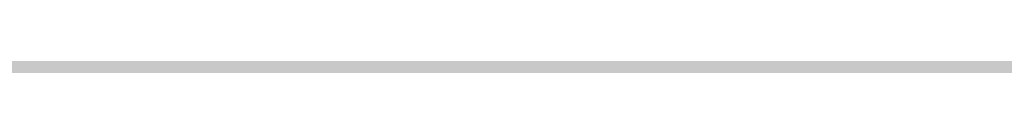
# Model space of a CAD drawing. Units: millimetres. Extents: x 0 to 2267, y 0 to 1823.
# Tile 181 of 256: x 1838.83 to 1841.442, y 1127.404 to 1127.414. Entities that reach past the tile are written whole.
import ezdxf

# ---------------------------------------------------------------- set-up
doc = ezdxf.new("R2010")
doc.units = ezdxf.units.MM
doc.header["$MEASUREMENT"] = 0
doc.layers.add('M-DIMS', color=2, linetype='Continuous', lineweight=25)
doc.layers.add('M-HATC', color=252, linetype='Continuous', lineweight=18)
doc.styles.get("Standard").update_dxf_attribs({"font": 'arial.ttf'})
doc.dimstyles.get("Standard").update_dxf_attribs({"dimtxt": 7, "dimasz": 4, "dimexe": 0.18, "dimexo": 0.0625, "dimgap": 0.09, "dimtad": 0, "dimdec": 0, "dimzin": 0, "dimdsep": 46, "dimtxsty": 'Standard', "dimcen": 0.09, "dimadec": 0, "dimazin": 0, "dimtfac": 1, "dimtdec": 0, "dimtofl": 0, "dimtmove": 0, "dimatfit": 3, "dimfxl": 1, "dimtolj": 1, "dimtzin": 0, "dimarcsym": 0})

# ---------------------------------------------------------------- blocks, each defined once
blk = doc.blocks.new('*D1')
at = {"layer": 'Defpoints', "color": 0, "transparency": 16777216}
for p in [(1593.4289, 1127.4171), (1843.4289, 1127.4171), (1843.4289, 955.6278)]:
    blk.add_point(p, dxfattribs=at)
at = {"layer": 'M-DIMS', "color": 0, "lineweight": -2, "transparency": 16777216}
for p, q in [((1593.4289, 1127.3546), (1593.4289, 955.4478)), ((1843.4289, 1127.3546), (1843.4289, 955.4478)), ((1597.4289, 955.6278), (1710.5582, 955.6278)), ((1839.4289, 955.6278), (1726.2996, 955.6278))]:
    blk.add_line(p, q, dxfattribs=at)
at = {"layer": 'M-DIMS', "color": 0, "transparency": 16777216}
for points in [[(1597.4289, 956.2944), (1597.4289, 954.9611), (1593.4289, 955.6278)], [(1839.4289, 956.2944), (1839.4289, 954.9611), (1843.4289, 955.6278)]]:
    blk.add_solid(points, dxfattribs=at)
at = {"layer": 'M-DIMS', "color": 0, "transparency": 16777216, "insert": (1718.4289, 955.6278), "char_height": 7, "attachment_point": 5}
blk.add_mtext('\\A1;250', dxfattribs=at)

msp = doc.modelspace()

# ---------------------------------------------------------------- hatches: boundary and pattern name
at = {"layer": 'M-HATC'}
h = msp.add_hatch(color=256, dxfattribs=at)
h.dxf.hatch_style = 1
h.paths.add_polyline_path([(2055.771, 1603.062), (1381.0868, 1603.062), (1381.0868, 1598.062), (2055.771, 1598.062)])
h.paths.add_polyline_path([(2055.771, 1598.062), (1381.0868, 1598.062), (1381.0868, 1593.062), (2055.771, 1593.062)])
h.paths.add_polyline_path([(2051.3074, 1536.7609), (1385.5504, 1536.7609), (1385.5504, 1526.7609), (1387.5504, 1526.7609), (1388.5366, 1525.0528), (1385.3319, 1521.2335), (1385.3319, 1521.2226), (2050.2542, 1522.7491), (2048.3212, 1525.0528), (2049.3074, 1526.7609), (2051.3074, 1526.7609)])
edge = h.paths.add_edge_path()
edge.add_arc((1847.5345, 1379.1492), 135, 222.603061, 222.890851, ccw=False)
edge.add_line((1748.1663, 1287.7656), (1683.0921, 1287.7656))
edge.add_arc((1583.7239, 1379.1492), 135, 317.109149, 317.396939, ccw=False)
edge.add_arc((1678.9686, 1290.6707), 5, 222.8909, 317.1091, ccw=False)
edge.add_arc((1774.2133, 1379.1492), 135, 222.603061, 222.890851, ccw=False)
edge.add_line((1674.8451, 1287.7656), (1609.7709, 1287.7656))
edge.add_arc((1510.4027, 1379.1492), 135, 317.109149, 317.396939, ccw=False)
edge.add_arc((1605.6474, 1290.6707), 5, 222.8909, 317.1091, ccw=False)
edge.add_arc((1700.8921, 1379.1492), 135, 222.603061, 222.890851, ccw=False)
edge.add_line((1601.5239, 1287.7656), (1536.4497, 1287.7656))
edge.add_arc((1437.0815, 1379.1492), 135, 317.109149, 317.396939, ccw=False)
edge.add_arc((1532.3262, 1290.6707), 5, 222.8909, 317.1091, ccw=False)
edge.add_arc((1627.5709, 1379.1492), 135, 222.603061, 222.890851, ccw=False)
edge.add_line((1528.2027, 1287.7656), (1505.9289, 1287.7656))
edge.add_spline(control_points=[(1505.9289, 1287.7656), (1504.2622, 1287.7656), (1504.2622, 1282.7656), (1505.9289, 1282.7656)], knot_values=[0, 0, 0, 0, 5, 5, 5, 5], degree=3, periodic=0)
edge.add_line((1505.9289, 1282.7656), (1930.9289, 1282.7656))
edge.add_spline(control_points=[(1930.9289, 1282.7656), (1932.5956, 1282.7656), (1932.5956, 1287.7656), (1930.9289, 1287.7656)], knot_values=[0, 0, 0, 0, 5, 5, 5, 5], degree=3, periodic=0)
edge.add_line((1930.9289, 1287.7656), (1903.0557, 1287.7656))
edge.add_arc((1803.6875, 1379.1492), 135, 317.109149, 317.396939, ccw=False)
edge.add_arc((1898.9322, 1290.6707), 5, 222.8909, 317.1091, ccw=False)
edge.add_arc((1994.1769, 1379.1492), 135, 222.603061, 222.890851, ccw=False)
edge.add_line((1894.8087, 1287.7656), (1829.7345, 1287.7656))
edge.add_arc((1730.3663, 1379.1492), 135, 317.109149, 317.396939, ccw=False)
edge.add_arc((1825.611, 1290.6707), 5, 222.8909, 317.1091, ccw=False)
edge.add_arc((1920.8557, 1379.1492), 135, 222.603061, 222.890851, ccw=False)
edge.add_line((1821.4875, 1287.7656), (1756.4133, 1287.7656))
edge.add_arc((1657.0451, 1379.1492), 135, 317.109149, 317.396939, ccw=False)
edge.add_arc((1752.2898, 1290.6707), 5, 222.8909, 317.1091, ccw=False)
edge = h.paths.add_edge_path()
edge.add_spline(control_points=[(1843.4289, 1227.2475), (1845.0956, 1227.2475), (1845.0956, 1232.2475), (1843.4289, 1232.2475)], knot_values=[0, 0, 0, 0, 5, 5, 5, 5], degree=3, periodic=0)
edge.add_line((1843.4289, 1232.2475), (1593.4289, 1232.2475))
edge.add_spline(control_points=[(1593.4289, 1232.2475), (1591.7622, 1232.2475), (1591.7622, 1227.2475), (1593.4289, 1227.2475)], knot_values=[0, 0, 0, 0, 5, 5, 5, 5], degree=3, periodic=0)
edge.add_line((1593.4289, 1227.2475), (1843.4289, 1227.2475))
h.paths.add_polyline_path([(1905.9289, 1127.4171), (1530.9289, 1127.4171, 0.414214), (1520.9289, 1117.4171), (1530.9289, 1117.4171), (1915.9289, 1117.4171, 0.414214)])
edge = h.paths.add_edge_path()
edge.add_arc((1397.0858, 1498.4078), 12.7299, 90.78215, 190.87871, ccw=False)
edge.add_line((1396.912, 1511.1365), (1428.0097, 1511.3488))
edge.add_line((1428.0097, 1511.3488), (1433.0097, 1511.3488))
edge.add_line((1433.0097, 1511.3488), (1434.439, 1511.3488))
edge.add_arc((1419.474, 1498.0804), 20, 41.561, 74.08211)
edge.add_line((1424.9592, 1517.3135), (1399.9351, 1517.2561))
edge.add_spline(control_points=[(1399.9307, 1517.2561), (1399.884, 1517.2131), (1399.8328, 1517.1689), (1399.7774, 1517.1236)], knot_values=[11.567499, 11.567499, 11.567499, 11.567499, 11.814249, 11.814249, 11.814249, 11.814249], degree=3, periodic=0)
edge.add_spline(control_points=[(1399.6328, 1517.0099), (1399.5831, 1516.9721), (1399.5307, 1516.9338), (1399.4759, 1516.8947)], knot_values=[11.167718, 11.167718, 11.167718, 11.167718, 11.365188, 11.365188, 11.365188, 11.365188], degree=3, periodic=0)
edge.add_spline(control_points=[(1399.3398, 1516.8001), (1399.1514, 1516.6719), (1398.9384, 1516.5377), (1398.704, 1516.3994)], knot_values=[10.376405, 10.376405, 10.376405, 10.376405, 11.00994, 11.00994, 11.00994, 11.00994], degree=3, periodic=0)
edge.add_spline(control_points=[(1398.6572, 1516.3719), (1398.5789, 1516.326), (1398.4983, 1516.2797), (1398.4155, 1516.2331)], knot_values=[10.125175, 10.125175, 10.125175, 10.125175, 10.334406, 10.334406, 10.334406, 10.334406], degree=3, periodic=0)
edge.add_spline(control_points=[(1398.2642, 1516.1487), (1398.196, 1516.1111), (1398.1263, 1516.0732), (1398.0555, 1516.0351)], knot_values=[9.832246, 9.832246, 9.832246, 9.832246, 9.999658, 9.999658, 9.999658, 9.999658], degree=3, periodic=0)
edge.add_spline(control_points=[(1397.9987, 1516.0048), (1397.7312, 1515.8621), (1397.446, 1515.7171), (1397.1466, 1515.5714)], knot_values=[9.161808, 9.161808, 9.161808, 9.161808, 9.787769, 9.787769, 9.787769, 9.787769], degree=3, periodic=0)
edge.add_spline(control_points=[(1397.1466, 1515.5714), (1396.8418, 1515.423), (1396.5222, 1515.274), (1396.1914, 1515.1262)], knot_values=[8.524455, 8.524455, 8.524455, 8.524455, 9.161808, 9.161808, 9.161808, 9.161808], degree=3, periodic=0)
edge.add_spline(control_points=[(1396.0777, 1515.0756), (1395.9854, 1515.0348), (1395.8922, 1514.994), (1395.7983, 1514.9534)], knot_values=[8.275193, 8.275193, 8.275193, 8.275193, 8.451726, 8.451726, 8.451726, 8.451726], degree=3, periodic=0)
edge.add_spline(control_points=[(1395.6018, 1514.8691), (1395.4997, 1514.8257), (1395.3968, 1514.7824), (1395.2932, 1514.7394)], knot_values=[7.962917, 7.962917, 7.962917, 7.962917, 8.152764, 8.152764, 8.152764, 8.152764], degree=3, periodic=0)
edge.add_spline(control_points=[(1395.2116, 1514.7057), (1394.8278, 1514.5475), (1394.4345, 1514.3929), (1394.0364, 1514.2442)], knot_values=[7.21254, 7.21254, 7.21254, 7.21254, 7.913148, 7.913148, 7.913148, 7.913148], degree=3, periodic=0)
edge.add_spline(control_points=[(1394.0364, 1514.2442), (1393.7076, 1514.1214), (1393.3754, 1514.0027), (1393.0427, 1513.8895)], knot_values=[6.633733, 6.633733, 6.633733, 6.633733, 7.21254, 7.21254, 7.21254, 7.21254], degree=3, periodic=0)
edge.add_spline(control_points=[(1392.8214, 1513.815), (1392.7198, 1513.7812), (1392.6181, 1513.7479), (1392.5166, 1513.7152)], knot_values=[6.328796, 6.328796, 6.328796, 6.328796, 6.505493, 6.505493, 6.505493, 6.505493], degree=3, periodic=0)
edge.add_spline(control_points=[(1392.5166, 1513.7152), (1392.3187, 1513.6515), (1392.1212, 1513.59), (1391.9244, 1513.531)], knot_values=[5.984605, 5.984605, 5.984605, 5.984605, 6.328796, 6.328796, 6.328796, 6.328796], degree=3, periodic=0)
edge.add_spline(control_points=[(1391.7915, 1513.4915), (1391.3122, 1513.3501), (1390.8384, 1513.2239), (1390.3784, 1513.1171)], knot_values=[5.066697, 5.066697, 5.066697, 5.066697, 5.907055, 5.907055, 5.907055, 5.907055], degree=3, periodic=0)
edge.add_spline(control_points=[(1390.3784, 1513.1171), (1390.1797, 1513.071), (1389.9836, 1513.0284), (1389.7907, 1512.9899)], knot_values=[4.70367, 4.70367, 4.70367, 4.70367, 5.066695, 5.066695, 5.066695, 5.066695], degree=3, periodic=0)
edge.add_spline(control_points=[(1389.422, 1512.9204), (1389.2459, 1512.8892), (1389.0729, 1512.8617), (1388.9036, 1512.8381)], knot_values=[4.130571, 4.130571, 4.130571, 4.130571, 4.469816, 4.469816, 4.469816, 4.469816], degree=3, periodic=0)
edge.add_spline(control_points=[(1388.9036, 1512.8381), (1388.591, 1512.7946), (1388.2911, 1512.7644), (1388.0071, 1512.7494)], knot_values=[3.504031, 3.504031, 3.504031, 3.504031, 4.130571, 4.130571, 4.130571, 4.130571], degree=3, periodic=0)
edge.add_spline(control_points=[(1387.9356, 1512.7459), (1387.8538, 1512.7423), (1387.7733, 1512.74), (1387.6944, 1512.739)], knot_values=[3.268866, 3.268866, 3.268866, 3.268866, 3.451164, 3.451164, 3.451164, 3.451164], degree=3, periodic=0)
edge.add_spline(control_points=[(1387.3351, 1512.7443), (1387.2076, 1512.7499), (1387.0847, 1512.7597), (1386.967, 1512.7739)], knot_values=[2.670686, 2.670686, 2.670686, 2.670686, 2.984, 2.984, 2.984, 2.984], degree=3, periodic=0)
edge.add_spline(control_points=[(1386.8327, 1512.7922), (1386.8209, 1512.7941), (1386.8092, 1512.7959), (1386.7975, 1512.7979)], knot_values=[2.516981, 2.516981, 2.516981, 2.516981, 2.549528, 2.549528, 2.549528, 2.549528], degree=3, periodic=0)
edge.add_spline(control_points=[(1386.4526, 1512.8735), (1386.4257, 1512.881), (1386.3993, 1512.889), (1386.3733, 1512.8972)], knot_values=[2.095869, 2.095869, 2.095869, 2.095869, 2.17941, 2.17941, 2.17941, 2.17941], degree=3, periodic=0)
edge.add_spline(control_points=[(1386.0691, 1513.0189), (1386.0634, 1513.0217), (1386.0577, 1513.0246), (1386.052, 1513.0275)], knot_values=[1.72453, 1.72453, 1.72453, 1.72453, 1.745933, 1.745933, 1.745933, 1.745933], degree=3, periodic=0)
edge.add_arc((1399.474, 1498.0804), 20, 131.82432, 180)
edge.add_arc((1630.3336, 1505.5484), 250.9708, 181.705176, 236.427975)
edge.add_arc((1605.3399, 1483.3044), 218.7822, 238.660829, 243.34961)
edge.add_arc((1647.0911, 1510.3592), 262.8986, 183.129836, 237.853442, ccw=False)
h.paths.add_polyline_path([(1406.5369, 1391.9644, 0.149382), (1491.5506, 1296.4418, -0.129517)], flags=17)
edge = h.paths.add_edge_path()
edge.add_arc((2037.3838, 1498.0804), 20, 0, 48.26587)
edge.add_spline(control_points=[(2050.6973, 1513.0052), (2050.6512, 1512.9847), (2050.6034, 1512.9655), (2050.5539, 1512.9477)], knot_values=[1.835652, 1.835652, 1.835652, 1.835652, 2.000781, 2.000781, 2.000781, 2.000781], degree=3, periodic=0)
edge.add_spline(control_points=[(2050.4616, 1512.9166), (2050.479, 1512.9221), (2050.4963, 1512.9277), (2050.5133, 1512.9335)], knot_values=[2.045477, 2.045477, 2.045477, 2.045477, 2.101389, 2.101389, 2.101389, 2.101389], degree=3, periodic=0)
edge.add_spline(control_points=[(2050.129, 1512.8342), (2050.1984, 1512.8473), (2050.2657, 1512.8623), (2050.3308, 1512.8792)], knot_values=[2.237629, 2.237629, 2.237629, 2.237629, 2.435841, 2.435841, 2.435841, 2.435841], degree=3, periodic=0)
edge.add_spline(control_points=[(2050.0946, 1512.8278), (2050.1061, 1512.8299), (2050.1176, 1512.832), (2050.129, 1512.8342)], knot_values=[2.435841, 2.435841, 2.435841, 2.435841, 2.468321, 2.468321, 2.468321, 2.468321], degree=3, periodic=0)
edge.add_spline(control_points=[(2049.7843, 1512.7851), (2049.8552, 1512.7922), (2049.9243, 1512.8008), (2049.9917, 1512.8109)], knot_values=[2.563852, 2.563852, 2.563852, 2.563852, 2.748541, 2.748541, 2.748541, 2.748541], degree=3, periodic=0)
edge.add_spline(control_points=[(2049.4052, 1512.7617), (2049.5364, 1512.7653), (2049.6629, 1512.773), (2049.7843, 1512.7851)], knot_values=[2.748541, 2.748541, 2.748541, 2.748541, 3.064882, 3.064882, 3.064882, 3.064882], degree=3, periodic=0)
edge.add_spline(control_points=[(2049.1698, 1512.7597), (2049.2336, 1512.7591), (2049.2965, 1512.7594), (2049.3584, 1512.7606)], knot_values=[3.102309, 3.102309, 3.102309, 3.102309, 3.2503, 3.2503, 3.2503, 3.2503], degree=3, periodic=0)
edge.add_spline(control_points=[(2048.8573, 1512.7691), (2048.9638, 1512.7638), (2049.068, 1512.7606), (2049.1698, 1512.7597)], knot_values=[3.2503, 3.2503, 3.2503, 3.2503, 3.486069, 3.486069, 3.486069, 3.486069], degree=3, periodic=0)
edge.add_spline(control_points=[(2048.6924, 1512.7789), (2048.3729, 1512.8009), (2048.0345, 1512.8411), (2047.6817, 1512.897)], knot_values=[3.606429, 3.606429, 3.606429, 3.606429, 4.2989, 4.2989, 4.2989, 4.2989], degree=3, periodic=0)
edge.add_spline(control_points=[(2047.6817, 1512.897), (2047.5458, 1512.9185), (2047.4077, 1512.9424), (2047.2678, 1512.9685)], knot_values=[4.2989, 4.2989, 4.2989, 4.2989, 4.565769, 4.565769, 4.565769, 4.565769], degree=3, periodic=0)
edge.add_spline(control_points=[(2047.2678, 1512.9685), (2047.1449, 1512.9914), (2047.0207, 1513.016), (2046.8951, 1513.0422)], knot_values=[4.565769, 4.565769, 4.565769, 4.565769, 4.799971, 4.799971, 4.799971, 4.799971], degree=3, periodic=0)
edge.add_spline(control_points=[(2046.8951, 1513.0422), (2046.5286, 1513.1188), (2046.1513, 1513.209), (2045.7676, 1513.3107)], knot_values=[4.799971, 4.799971, 4.799971, 4.799971, 5.483718, 5.483718, 5.483718, 5.483718], degree=3, periodic=0)
edge.add_spline(control_points=[(2045.7676, 1513.3107), (2045.3724, 1513.4154), (2044.9704, 1513.5322), (2044.5662, 1513.6588)], knot_values=[5.483718, 5.483718, 5.483718, 5.483718, 6.187866, 6.187866, 6.187866, 6.187866], degree=3, periodic=0)
edge.add_spline(control_points=[(2044.5662, 1513.6588), (2044.4149, 1513.7061), (2044.2633, 1513.7549), (2044.1116, 1513.8048)], knot_values=[6.187866, 6.187866, 6.187866, 6.187866, 6.451551, 6.451551, 6.451551, 6.451551], degree=3, periodic=0)
edge.add_spline(control_points=[(2044.1116, 1513.8048), (2043.9967, 1513.8427), (2043.8817, 1513.8813), (2043.7668, 1513.9205)], knot_values=[6.451551, 6.451551, 6.451551, 6.451551, 6.651434, 6.651434, 6.651434, 6.651434], degree=3, periodic=0)
edge.add_spline(control_points=[(2043.7668, 1513.9205), (2043.3716, 1514.0554), (2042.9774, 1514.1979), (2042.5886, 1514.3458)], knot_values=[6.651434, 6.651434, 6.651434, 6.651434, 7.338879, 7.338879, 7.338879, 7.338879], degree=3, periodic=0)
edge.add_spline(control_points=[(2042.5886, 1514.3458), (2042.1643, 1514.5071), (2041.7465, 1514.6749), (2041.3409, 1514.846)], knot_values=[7.338879, 7.338879, 7.338879, 7.338879, 8.089209, 8.089209, 8.089209, 8.089209], degree=3, periodic=0)
edge.add_spline(control_points=[(2041.3409, 1514.846), (2041.1028, 1514.9465), (2040.869, 1515.0481), (2040.6405, 1515.1502)], knot_values=[8.089209, 8.089209, 8.089209, 8.089209, 8.529587, 8.529587, 8.529587, 8.529587], degree=3, periodic=0)
edge.add_spline(control_points=[(2040.51, 1515.2089), (2040.0824, 1515.4022), (2039.6747, 1515.5971), (2039.295, 1515.7894)], knot_values=[8.613818, 8.613818, 8.613818, 8.613818, 9.44571, 9.44571, 9.44571, 9.44571], degree=3, periodic=0)
edge.add_spline(control_points=[(2039.295, 1515.7894), (2039.0618, 1515.9075), (2038.8391, 1516.0246), (2038.6288, 1516.1398)], knot_values=[9.44571, 9.44571, 9.44571, 9.44571, 9.956404, 9.956404, 9.956404, 9.956404], degree=3, periodic=0)
edge.add_spline(control_points=[(2038.6288, 1516.1398), (2038.5187, 1516.2001), (2038.4121, 1516.2598), (2038.309, 1516.3189)], knot_values=[9.956404, 9.956404, 9.956404, 9.956404, 10.223542, 10.223542, 10.223542, 10.223542], degree=3, periodic=0)
edge.add_spline(control_points=[(2038.309, 1516.3189), (2038.2138, 1516.3735), (2038.1216, 1516.4276), (2038.0328, 1516.481)], knot_values=[10.223542, 10.223542, 10.223542, 10.223542, 10.47051, 10.47051, 10.47051, 10.47051], degree=3, periodic=0)
edge.add_spline(control_points=[(2038.0328, 1516.481), (2037.7855, 1516.6296), (2037.5639, 1516.773), (2037.3722, 1516.909)], knot_values=[10.47051, 10.47051, 10.47051, 10.47051, 11.15767, 11.15767, 11.15767, 11.15767], degree=3, periodic=0)
edge.add_spline(control_points=[(2037.3722, 1516.909), (2037.2789, 1516.9752), (2037.1927, 1517.0396), (2037.1142, 1517.102)], knot_values=[11.15767, 11.15767, 11.15767, 11.15767, 11.49227, 11.49227, 11.49227, 11.49227], degree=3, periodic=0)
edge.add_spline(control_points=[(2036.8564, 1517.3259), (2036.9148, 1517.2692), (2036.9814, 1517.2103), (2037.0557, 1517.1492)], knot_values=[11.577341, 11.577341, 11.577341, 11.577341, 11.91035, 11.91035, 11.91035, 11.91035], degree=3, periodic=0)
edge.add_spline(control_points=[(2036.8074, 1517.3748), (2036.823, 1517.3587), (2036.8393, 1517.3424), (2036.8564, 1517.3259)], knot_values=[11.91035, 11.91035, 11.91035, 11.91035, 12.007402, 12.007402, 12.007402, 12.007402], degree=3, periodic=0)
edge.add_spline(control_points=[(2036.7017, 1517.494), (2036.7104, 1517.483), (2036.7196, 1517.4719), (2036.7291, 1517.4606)], knot_values=[12.184155, 12.184155, 12.184155, 12.184155, 12.255409, 12.255409, 12.255409, 12.255409], degree=3, periodic=0)
edge.add_spline(control_points=[(2036.6159, 1517.6205), (2036.62, 1517.613), (2036.6243, 1517.6055), (2036.6289, 1517.5979)], knot_values=[12.487913, 12.487913, 12.487913, 12.487913, 12.541035, 12.541035, 12.541035, 12.541035], degree=3, periodic=0)
edge.add_spline(control_points=[(2036.5635, 1517.786), (2036.5637, 1517.7794), (2036.5642, 1517.7726), (2036.565, 1517.7658)], knot_values=[12.911761, 12.911761, 12.911761, 12.911761, 12.968286, 12.968286, 12.968286, 12.968286], degree=3, periodic=0)
edge.add_spline(control_points=[(2036.6166, 1517.9304), (2036.6125, 1517.9259), (2036.6086, 1517.9212), (2036.6049, 1517.9165)], knot_values=[13.382527, 13.382527, 13.382527, 13.382527, 13.433791, 13.433791, 13.433791, 13.433791], degree=3, periodic=0)
edge.add_spline(control_points=[(2036.749, 1518.017), (2036.7361, 1518.0116), (2036.7239, 1518.006), (2036.7124, 1518.0002)], knot_values=[13.726299, 13.726299, 13.726299, 13.726299, 13.809928, 13.809928, 13.809928, 13.809928], degree=3, periodic=0)
edge.add_spline(control_points=[(2036.8604, 1518.0528), (2036.8386, 1518.0474), (2036.8181, 1518.0416), (2036.7988, 1518.0353)], knot_values=[13.910887, 13.910887, 13.910887, 13.910887, 14.02153, 14.02153, 14.02153, 14.02153], degree=3, periodic=0)
edge.add_line((2036.9639, 1518.0804), (2032.3838, 1518.0804))
edge.add_line((2032.3838, 1518.0804), (2027.3838, 1518.0804))
edge.add_line((2027.3838, 1518.0804), (2022.3838, 1518.0804))
edge.add_line((2022.3838, 1518.0804), (2017.3838, 1518.0804))
edge.add_arc((2017.3838, 1498.0804), 20, 90, 138.439)
edge.add_line((2002.4188, 1511.3488), (2003.8481, 1511.3488))
edge.add_line((2003.8481, 1511.3488), (2008.8481, 1511.3488))
edge.add_line((2008.8481, 1511.3488), (2039.772, 1511.1377))
edge.add_arc((2039.772, 1498.4078), 12.7299, -10.87871, 90, ccw=False)
edge.add_arc((1789.7668, 1510.3592), 262.8986, 302.146558, 356.870164, ccw=False)
edge.add_arc((1831.5179, 1483.3044), 218.7822, 296.65039, 301.339171)
edge.add_arc((1806.5242, 1505.5484), 250.9708, 303.572025, 358.294824)
h.paths.add_polyline_path([(2030.321, 1391.9644, -0.129517), (1945.3072, 1296.4418, 0.149382)], flags=17)
edge = h.paths.add_edge_path()
edge.add_spline(control_points=[(2037.2464, 1518.0821), (2037.2898, 1518.081), (2037.3355, 1518.0804), (2037.3838, 1518.0804)], knot_values=[0.000012, 0.000012, 0.000012, 0.000012, 0.144754, 0.144754, 0.144754, 0.144754], degree=3, periodic=0)
edge.add_line((2037.3357, 1518.0804), (2037.0096, 1518.0804))
edge.add_spline(control_points=[(2037.0096, 1518.0804), (2036.9822, 1518.0768), (2036.956, 1518.0727), (2036.9312, 1518.0681)], knot_values=[14.13465, 14.13465, 14.13465, 14.13465, 14.247197, 14.247197, 14.247197, 14.247197], degree=3, periodic=0)
edge.add_spline(control_points=[(2036.9312, 1518.0681), (2036.9276, 1518.0674), (2036.9241, 1518.0667), (2036.9205, 1518.0661)], knot_values=[14.118315, 14.118315, 14.118315, 14.118315, 14.13465, 14.13465, 14.13465, 14.13465], degree=3, periodic=0)
edge.add_spline(control_points=[(2036.9205, 1518.0661), (2036.9118, 1518.0644), (2036.9032, 1518.0626), (2036.8948, 1518.0608)], knot_values=[14.078086, 14.078086, 14.078086, 14.078086, 14.118315, 14.118315, 14.118315, 14.118315], degree=3, periodic=0)
edge.add_spline(control_points=[(2036.8948, 1518.0608), (2036.883, 1518.0583), (2036.8716, 1518.0556), (2036.8604, 1518.0528)], knot_values=[14.02153, 14.02153, 14.02153, 14.02153, 14.078086, 14.078086, 14.078086, 14.078086], degree=3, periodic=0)
edge.add_spline(control_points=[(2036.8604, 1518.0528), (2036.8386, 1518.0474), (2036.8181, 1518.0416), (2036.7988, 1518.0353)], knot_values=[13.910887, 13.910887, 13.910887, 13.910887, 14.02153, 14.02153, 14.02153, 14.02153], degree=3, periodic=0)
edge.add_spline(control_points=[(2036.7988, 1518.0353), (2036.7981, 1518.035), (2036.7974, 1518.0348), (2036.7967, 1518.0346)], knot_values=[13.906906, 13.906906, 13.906906, 13.906906, 13.910887, 13.910887, 13.910887, 13.910887], degree=3, periodic=0)
edge.add_spline(control_points=[(2036.7967, 1518.0346), (2036.7882, 1518.0318), (2036.7799, 1518.0289), (2036.7719, 1518.0259)], knot_values=[13.857826, 13.857826, 13.857826, 13.857826, 13.906906, 13.906906, 13.906906, 13.906906], degree=3, periodic=0)
edge.add_spline(control_points=[(2036.7719, 1518.0259), (2036.764, 1518.023), (2036.7564, 1518.02), (2036.749, 1518.017)], knot_values=[13.809928, 13.809928, 13.809928, 13.809928, 13.857826, 13.857826, 13.857826, 13.857826], degree=3, periodic=0)
edge.add_spline(control_points=[(2036.749, 1518.017), (2036.7361, 1518.0116), (2036.7239, 1518.006), (2036.7124, 1518.0002)], knot_values=[13.726299, 13.726299, 13.726299, 13.726299, 13.809928, 13.809928, 13.809928, 13.809928], degree=3, periodic=0)
edge.add_spline(control_points=[(2036.7124, 1518.0002), (2036.7121, 1518), (2036.7118, 1517.9999), (2036.7115, 1517.9997)], knot_values=[13.723993, 13.723993, 13.723993, 13.723993, 13.726299, 13.726299, 13.726299, 13.726299], degree=3, periodic=0)
edge.add_spline(control_points=[(2036.7115, 1517.9997), (2036.7063, 1517.9971), (2036.7013, 1517.9944), (2036.6965, 1517.9917)], knot_values=[13.686536, 13.686536, 13.686536, 13.686536, 13.723993, 13.723993, 13.723993, 13.723993], degree=3, periodic=0)
edge.add_spline(control_points=[(2036.6965, 1517.9917), (2036.6919, 1517.9891), (2036.6874, 1517.9865), (2036.6831, 1517.9839)], knot_values=[13.651251, 13.651251, 13.651251, 13.651251, 13.686536, 13.686536, 13.686536, 13.686536], degree=3, periodic=0)
edge.add_spline(control_points=[(2036.6831, 1517.9839), (2036.6764, 1517.9798), (2036.67, 1517.9757), (2036.6639, 1517.9714)], knot_values=[13.596804, 13.596804, 13.596804, 13.596804, 13.651251, 13.651251, 13.651251, 13.651251], degree=3, periodic=0)
edge.add_spline(control_points=[(2036.6639, 1517.9714), (2036.6636, 1517.9712), (2036.6633, 1517.9709), (2036.6629, 1517.9707)], knot_values=[13.593956, 13.593956, 13.593956, 13.593956, 13.596804, 13.596804, 13.596804, 13.596804], degree=3, periodic=0)
edge.add_spline(control_points=[(2036.6629, 1517.9707), (2036.6603, 1517.9689), (2036.6577, 1517.967), (2036.6552, 1517.9651)], knot_values=[13.570322, 13.570322, 13.570322, 13.570322, 13.593956, 13.593956, 13.593956, 13.593956], degree=3, periodic=0)
edge.add_spline(control_points=[(2036.6552, 1517.9651), (2036.6525, 1517.9631), (2036.6499, 1517.9611), (2036.6474, 1517.9591)], knot_values=[13.545477, 13.545477, 13.545477, 13.545477, 13.570322, 13.570322, 13.570322, 13.570322], degree=3, periodic=0)
edge.add_spline(control_points=[(2036.6474, 1517.9591), (2036.6472, 1517.9589), (2036.6471, 1517.9588), (2036.6469, 1517.9587)], knot_values=[13.543931, 13.543931, 13.543931, 13.543931, 13.545477, 13.545477, 13.545477, 13.545477], degree=3, periodic=0)
edge.add_spline(control_points=[(2036.6469, 1517.9587), (2036.6412, 1517.9541), (2036.6358, 1517.9494), (2036.6307, 1517.9447)], knot_values=[13.488237, 13.488237, 13.488237, 13.488237, 13.543931, 13.543931, 13.543931, 13.543931], degree=3, periodic=0)
edge.add_spline(control_points=[(2036.6307, 1517.9447), (2036.6282, 1517.9423), (2036.6257, 1517.9399), (2036.6233, 1517.9374)], knot_values=[13.460307, 13.460307, 13.460307, 13.460307, 13.488237, 13.488237, 13.488237, 13.488237], degree=3, periodic=0)
edge.add_spline(control_points=[(2036.6233, 1517.9374), (2036.6215, 1517.9356), (2036.6198, 1517.9338), (2036.6181, 1517.932)], knot_values=[13.439712, 13.439712, 13.439712, 13.439712, 13.460307, 13.460307, 13.460307, 13.460307], degree=3, periodic=0)
edge.add_spline(control_points=[(2036.6181, 1517.932), (2036.6176, 1517.9315), (2036.6171, 1517.9309), (2036.6166, 1517.9304)], knot_values=[13.433791, 13.433791, 13.433791, 13.433791, 13.439712, 13.439712, 13.439712, 13.439712], degree=3, periodic=0)
edge.add_spline(control_points=[(2036.6166, 1517.9304), (2036.6125, 1517.9259), (2036.6086, 1517.9212), (2036.6049, 1517.9165)], knot_values=[13.382527, 13.382527, 13.382527, 13.382527, 13.433791, 13.433791, 13.433791, 13.433791], degree=3, periodic=0)
edge.add_spline(control_points=[(2036.6049, 1517.9165), (2036.6026, 1517.9135), (2036.6004, 1517.9104), (2036.5982, 1517.9074)], knot_values=[13.350017, 13.350017, 13.350017, 13.350017, 13.382527, 13.382527, 13.382527, 13.382527], degree=3, periodic=0)
edge.add_spline(control_points=[(2036.5982, 1517.9074), (2036.5972, 1517.9059), (2036.5962, 1517.9043), (2036.5952, 1517.9028)], knot_values=[13.333922, 13.333922, 13.333922, 13.333922, 13.350017, 13.350017, 13.350017, 13.350017], degree=3, periodic=0)
edge.add_spline(control_points=[(2036.5952, 1517.9028), (2036.5945, 1517.9018), (2036.5939, 1517.9009), (2036.5933, 1517.8999)], knot_values=[13.323828, 13.323828, 13.323828, 13.323828, 13.333922, 13.333922, 13.333922, 13.333922], degree=3, periodic=0)
edge.add_spline(control_points=[(2036.5933, 1517.8999), (2036.5905, 1517.8955), (2036.5879, 1517.8909), (2036.5855, 1517.8864)], knot_values=[13.277545, 13.277545, 13.277545, 13.277545, 13.323828, 13.323828, 13.323828, 13.323828], degree=3, periodic=0)
edge.add_spline(control_points=[(2036.5855, 1517.8864), (2036.5836, 1517.8827), (2036.5817, 1517.8789), (2036.5801, 1517.8751)], knot_values=[13.240119, 13.240119, 13.240119, 13.240119, 13.277545, 13.277545, 13.277545, 13.277545], degree=3, periodic=0)
edge.add_spline(control_points=[(2036.5801, 1517.8751), (2036.5795, 1517.8739), (2036.579, 1517.8727), (2036.5785, 1517.8715)], knot_values=[13.228211, 13.228211, 13.228211, 13.228211, 13.240119, 13.240119, 13.240119, 13.240119], degree=3, periodic=0)
edge.add_spline(control_points=[(2036.5785, 1517.8715), (2036.578, 1517.8702), (2036.5774, 1517.869), (2036.5769, 1517.8677)], knot_values=[13.215717, 13.215717, 13.215717, 13.215717, 13.228211, 13.228211, 13.228211, 13.228211], degree=3, periodic=0)
edge.add_spline(control_points=[(2036.5769, 1517.8677), (2036.5755, 1517.864), (2036.5741, 1517.8603), (2036.5729, 1517.8565)], knot_values=[13.179847, 13.179847, 13.179847, 13.179847, 13.215717, 13.215717, 13.215717, 13.215717], degree=3, periodic=0)
edge.add_spline(control_points=[(2036.5729, 1517.8565), (2036.5713, 1517.8515), (2036.5699, 1517.8464), (2036.5687, 1517.8413)], knot_values=[13.132017, 13.132017, 13.132017, 13.132017, 13.179847, 13.179847, 13.179847, 13.179847], degree=3, periodic=0)
edge.add_spline(control_points=[(2036.5687, 1517.8413), (2036.5684, 1517.8402), (2036.5682, 1517.8392), (2036.568, 1517.8382)], knot_values=[13.122482, 13.122482, 13.122482, 13.122482, 13.132017, 13.132017, 13.132017, 13.132017], degree=3, periodic=0)
edge.add_spline(control_points=[(2036.568, 1517.8382), (2036.5676, 1517.8363), (2036.5672, 1517.8345), (2036.5669, 1517.8327)], knot_values=[13.105592, 13.105592, 13.105592, 13.105592, 13.122482, 13.122482, 13.122482, 13.122482], degree=3, periodic=0)
edge.add_spline(control_points=[(2036.5669, 1517.8327), (2036.5662, 1517.8292), (2036.5657, 1517.8257), (2036.5652, 1517.8222)], knot_values=[13.074063, 13.074063, 13.074063, 13.074063, 13.105592, 13.105592, 13.105592, 13.105592], degree=3, periodic=0)
edge.add_spline(control_points=[(2036.5652, 1517.8222), (2036.5652, 1517.8222), (2036.5652, 1517.8222), (2036.5652, 1517.8222)], knot_values=[13.074043, 13.074043, 13.074043, 13.074043, 13.074063, 13.074063, 13.074063, 13.074063], degree=3, periodic=0)
edge.add_spline(control_points=[(2036.5652, 1517.8222), (2036.5644, 1517.8164), (2036.5639, 1517.8106), (2036.5636, 1517.8046)], knot_values=[13.021884, 13.021884, 13.021884, 13.021884, 13.074043, 13.074043, 13.074043, 13.074043], degree=3, periodic=0)
edge.add_spline(control_points=[(2036.5636, 1517.8046), (2036.5636, 1517.804), (2036.5636, 1517.8034), (2036.5635, 1517.8028)], knot_values=[13.01674, 13.01674, 13.01674, 13.01674, 13.021884, 13.021884, 13.021884, 13.021884], degree=3, periodic=0)
edge.add_spline(control_points=[(2036.5635, 1517.8028), (2036.5634, 1517.8005), (2036.5634, 1517.7982), (2036.5634, 1517.7958)], knot_values=[12.996438, 12.996438, 12.996438, 12.996438, 13.01674, 13.01674, 13.01674, 13.01674], degree=3, periodic=0)
edge.add_spline(control_points=[(2036.5634, 1517.7958), (2036.5633, 1517.7926), (2036.5634, 1517.7893), (2036.5635, 1517.786)], knot_values=[12.968286, 12.968286, 12.968286, 12.968286, 12.996438, 12.996438, 12.996438, 12.996438], degree=3, periodic=0)
edge.add_spline(control_points=[(2036.5635, 1517.786), (2036.5637, 1517.7794), (2036.5642, 1517.7726), (2036.565, 1517.7658)], knot_values=[12.911761, 12.911761, 12.911761, 12.911761, 12.968286, 12.968286, 12.968286, 12.968286], degree=3, periodic=0)
edge.add_spline(control_points=[(2036.565, 1517.7658), (2036.565, 1517.7657), (2036.565, 1517.7656), (2036.565, 1517.7656)], knot_values=[12.911017, 12.911017, 12.911017, 12.911017, 12.911761, 12.911761, 12.911761, 12.911761], degree=3, periodic=0)
edge.add_spline(control_points=[(2036.565, 1517.7656), (2036.5654, 1517.7625), (2036.5658, 1517.7593), (2036.5663, 1517.7562)], knot_values=[12.88528, 12.88528, 12.88528, 12.88528, 12.911017, 12.911017, 12.911017, 12.911017], degree=3, periodic=0)
edge.add_spline(control_points=[(2036.5663, 1517.7562), (2036.5667, 1517.7534), (2036.5672, 1517.7506), (2036.5677, 1517.7478)], knot_values=[12.862519, 12.862519, 12.862519, 12.862519, 12.88528, 12.88528, 12.88528, 12.88528], degree=3, periodic=0)
edge.add_spline(control_points=[(2036.5677, 1517.7478), (2036.5678, 1517.7474), (2036.5679, 1517.7469), (2036.568, 1517.7465)], knot_values=[12.858885, 12.858885, 12.858885, 12.858885, 12.862519, 12.862519, 12.862519, 12.862519], degree=3, periodic=0)
edge.add_spline(control_points=[(2036.568, 1517.7465), (2036.5692, 1517.7399), (2036.5707, 1517.7332), (2036.5724, 1517.7264)], knot_values=[12.8053, 12.8053, 12.8053, 12.8053, 12.858885, 12.858885, 12.858885, 12.858885], degree=3, periodic=0)
edge.add_spline(control_points=[(2036.5724, 1517.7264), (2036.5734, 1517.7226), (2036.5745, 1517.7187), (2036.5756, 1517.7149)], knot_values=[12.775176, 12.775176, 12.775176, 12.775176, 12.8053, 12.8053, 12.8053, 12.8053], degree=3, periodic=0)
edge.add_spline(control_points=[(2036.5756, 1517.7149), (2036.5763, 1517.7125), (2036.577, 1517.7102), (2036.5778, 1517.7078)], knot_values=[12.756759, 12.756759, 12.756759, 12.756759, 12.775176, 12.775176, 12.775176, 12.775176], degree=3, periodic=0)
edge.add_spline(control_points=[(2036.5778, 1517.7078), (2036.5781, 1517.7067), (2036.5784, 1517.7057), (2036.5787, 1517.7047)], knot_values=[12.748742, 12.748742, 12.748742, 12.748742, 12.756759, 12.756759, 12.756759, 12.756759], degree=3, periodic=0)
edge.add_spline(control_points=[(2036.5787, 1517.7047), (2036.5808, 1517.6983), (2036.5831, 1517.6919), (2036.5856, 1517.6854)], knot_values=[12.69959, 12.69959, 12.69959, 12.69959, 12.748742, 12.748742, 12.748742, 12.748742], degree=3, periodic=0)
edge.add_spline(control_points=[(2036.5856, 1517.6854), (2036.5876, 1517.68), (2036.5898, 1517.6746), (2036.5921, 1517.6692)], knot_values=[12.659038, 12.659038, 12.659038, 12.659038, 12.69959, 12.69959, 12.69959, 12.69959], degree=3, periodic=0)
edge.add_spline(control_points=[(2036.5921, 1517.6692), (2036.594, 1517.6648), (2036.5959, 1517.6605), (2036.5979, 1517.6561)], knot_values=[12.626806, 12.626806, 12.626806, 12.626806, 12.659038, 12.659038, 12.659038, 12.659038], degree=3, periodic=0)
edge.add_spline(control_points=[(2036.5979, 1517.6561), (2036.5984, 1517.6551), (2036.5989, 1517.6541), (2036.5993, 1517.6531)], knot_values=[12.619394, 12.619394, 12.619394, 12.619394, 12.626806, 12.626806, 12.626806, 12.626806], degree=3, periodic=0)
edge.add_spline(control_points=[(2036.5993, 1517.6531), (2036.6043, 1517.6424), (2036.6099, 1517.6315), (2036.6159, 1517.6205)], knot_values=[12.541039, 12.541039, 12.541039, 12.541039, 12.619394, 12.619394, 12.619394, 12.619394], degree=3, periodic=0)
edge.add_spline(control_points=[(2036.6159, 1517.6205), (2036.6159, 1517.6205), (2036.6159, 1517.6205), (2036.6159, 1517.6205)], knot_values=[12.541035, 12.541035, 12.541035, 12.541035, 12.541039, 12.541039, 12.541039, 12.541039], degree=3, periodic=0)
edge.add_spline(control_points=[(2036.6159, 1517.6205), (2036.62, 1517.613), (2036.6243, 1517.6055), (2036.6289, 1517.5979)], knot_values=[12.487913, 12.487913, 12.487913, 12.487913, 12.541035, 12.541035, 12.541035, 12.541035], degree=3, periodic=0)
edge.add_spline(control_points=[(2036.6289, 1517.5979), (2036.6326, 1517.5916), (2036.6365, 1517.5853), (2036.6406, 1517.5789)], knot_values=[12.443982, 12.443982, 12.443982, 12.443982, 12.487913, 12.487913, 12.487913, 12.487913], degree=3, periodic=0)
edge.add_spline(control_points=[(2036.6406, 1517.5789), (2036.6414, 1517.5776), (2036.6423, 1517.5763), (2036.6431, 1517.5749)], knot_values=[12.434996, 12.434996, 12.434996, 12.434996, 12.443982, 12.443982, 12.443982, 12.443982], degree=3, periodic=0)
edge.add_spline(control_points=[(2036.6431, 1517.5749), (2036.6531, 1517.5596), (2036.6639, 1517.5439), (2036.6756, 1517.528)], knot_values=[12.329647, 12.329647, 12.329647, 12.329647, 12.434996, 12.434996, 12.434996, 12.434996], degree=3, periodic=0)
edge.add_spline(control_points=[(2036.6756, 1517.528), (2036.6839, 1517.5168), (2036.6925, 1517.5055), (2036.7017, 1517.494)], knot_values=[12.255409, 12.255409, 12.255409, 12.255409, 12.329647, 12.329647, 12.329647, 12.329647], degree=3, periodic=0)
edge.add_spline(control_points=[(2036.7017, 1517.494), (2036.7104, 1517.483), (2036.7196, 1517.4719), (2036.7291, 1517.4606)], knot_values=[12.184155, 12.184155, 12.184155, 12.184155, 12.255409, 12.255409, 12.255409, 12.255409], degree=3, periodic=0)
edge.add_spline(control_points=[(2036.7291, 1517.4606), (2036.7436, 1517.4435), (2036.759, 1517.4262), (2036.7753, 1517.4085)], knot_values=[12.075961, 12.075961, 12.075961, 12.075961, 12.184155, 12.184155, 12.184155, 12.184155], degree=3, periodic=0)
edge.add_spline(control_points=[(2036.7753, 1517.4085), (2036.7763, 1517.4075), (2036.7773, 1517.4064), (2036.7783, 1517.4054)], knot_values=[12.069502, 12.069502, 12.069502, 12.069502, 12.075961, 12.075961, 12.075961, 12.075961], degree=3, periodic=0)
edge.add_spline(control_points=[(2036.7783, 1517.4054), (2036.7877, 1517.3953), (2036.7974, 1517.385), (2036.8074, 1517.3748)], knot_values=[12.007402, 12.007402, 12.007402, 12.007402, 12.069502, 12.069502, 12.069502, 12.069502], degree=3, periodic=0)
edge.add_spline(control_points=[(2036.8074, 1517.3748), (2036.823, 1517.3587), (2036.8393, 1517.3424), (2036.8564, 1517.3259)], knot_values=[11.91035, 11.91035, 11.91035, 11.91035, 12.007402, 12.007402, 12.007402, 12.007402], degree=3, periodic=0)
edge.add_spline(control_points=[(2036.8564, 1517.3259), (2036.9148, 1517.2692), (2036.9814, 1517.2103), (2037.0557, 1517.1492)], knot_values=[11.577341, 11.577341, 11.577341, 11.577341, 11.91035, 11.91035, 11.91035, 11.91035], degree=3, periodic=0)
edge.add_spline(control_points=[(2037.0557, 1517.1492), (2037.0747, 1517.1336), (2037.0942, 1517.1179), (2037.1142, 1517.102)], knot_values=[11.49227, 11.49227, 11.49227, 11.49227, 11.577341, 11.577341, 11.577341, 11.577341], degree=3, periodic=0)
edge.add_spline(control_points=[(2037.1142, 1517.102), (2037.1927, 1517.0396), (2037.2789, 1516.9752), (2037.3722, 1516.909)], knot_values=[11.15767, 11.15767, 11.15767, 11.15767, 11.49227, 11.49227, 11.49227, 11.49227], degree=3, periodic=0)
edge.add_spline(control_points=[(2037.3722, 1516.909), (2037.5639, 1516.773), (2037.7855, 1516.6296), (2038.0328, 1516.481)], knot_values=[10.47051, 10.47051, 10.47051, 10.47051, 11.15767, 11.15767, 11.15767, 11.15767], degree=3, periodic=0)
edge.add_spline(control_points=[(2038.0328, 1516.481), (2038.1216, 1516.4276), (2038.2138, 1516.3735), (2038.309, 1516.3189)], knot_values=[10.223542, 10.223542, 10.223542, 10.223542, 10.47051, 10.47051, 10.47051, 10.47051], degree=3, periodic=0)
edge.add_spline(control_points=[(2038.309, 1516.3189), (2038.4121, 1516.2598), (2038.5187, 1516.2001), (2038.6288, 1516.1398)], knot_values=[9.956404, 9.956404, 9.956404, 9.956404, 10.223542, 10.223542, 10.223542, 10.223542], degree=3, periodic=0)
edge.add_spline(control_points=[(2038.6288, 1516.1398), (2038.8391, 1516.0246), (2039.0618, 1515.9075), (2039.295, 1515.7894)], knot_values=[9.44571, 9.44571, 9.44571, 9.44571, 9.956404, 9.956404, 9.956404, 9.956404], degree=3, periodic=0)
edge.add_spline(control_points=[(2039.295, 1515.7894), (2039.6747, 1515.5971), (2040.0824, 1515.4022), (2040.51, 1515.2089)], knot_values=[8.613818, 8.613818, 8.613818, 8.613818, 9.44571, 9.44571, 9.44571, 9.44571], degree=3, periodic=0)
edge.add_spline(control_points=[(2040.51, 1515.2089), (2040.5533, 1515.1893), (2040.5968, 1515.1697), (2040.6405, 1515.1502)], knot_values=[8.529587, 8.529587, 8.529587, 8.529587, 8.613818, 8.613818, 8.613818, 8.613818], degree=3, periodic=0)
edge.add_spline(control_points=[(2040.6405, 1515.1502), (2040.869, 1515.0481), (2041.1028, 1514.9465), (2041.3409, 1514.846)], knot_values=[8.089209, 8.089209, 8.089209, 8.089209, 8.529587, 8.529587, 8.529587, 8.529587], degree=3, periodic=0)
edge.add_spline(control_points=[(2041.3409, 1514.846), (2041.7465, 1514.6749), (2042.1643, 1514.5071), (2042.5886, 1514.3458)], knot_values=[7.338879, 7.338879, 7.338879, 7.338879, 8.089209, 8.089209, 8.089209, 8.089209], degree=3, periodic=0)
edge.add_spline(control_points=[(2042.5886, 1514.3458), (2042.9774, 1514.1979), (2043.3716, 1514.0554), (2043.7668, 1513.9205)], knot_values=[6.651434, 6.651434, 6.651434, 6.651434, 7.338879, 7.338879, 7.338879, 7.338879], degree=3, periodic=0)
edge.add_spline(control_points=[(2043.7668, 1513.9205), (2043.8817, 1513.8813), (2043.9967, 1513.8427), (2044.1116, 1513.8048)], knot_values=[6.451551, 6.451551, 6.451551, 6.451551, 6.651434, 6.651434, 6.651434, 6.651434], degree=3, periodic=0)
edge.add_spline(control_points=[(2044.1116, 1513.8048), (2044.2633, 1513.7549), (2044.4149, 1513.7061), (2044.5662, 1513.6588)], knot_values=[6.187866, 6.187866, 6.187866, 6.187866, 6.451551, 6.451551, 6.451551, 6.451551], degree=3, periodic=0)
edge.add_spline(control_points=[(2044.5662, 1513.6588), (2044.9704, 1513.5322), (2045.3724, 1513.4154), (2045.7676, 1513.3107)], knot_values=[5.483718, 5.483718, 5.483718, 5.483718, 6.187866, 6.187866, 6.187866, 6.187866], degree=3, periodic=0)
edge.add_spline(control_points=[(2045.7676, 1513.3107), (2046.1513, 1513.209), (2046.5286, 1513.1188), (2046.8951, 1513.0422)], knot_values=[4.799971, 4.799971, 4.799971, 4.799971, 5.483718, 5.483718, 5.483718, 5.483718], degree=3, periodic=0)
edge.add_spline(control_points=[(2046.8951, 1513.0422), (2047.0207, 1513.016), (2047.1449, 1512.9914), (2047.2678, 1512.9685)], knot_values=[4.565769, 4.565769, 4.565769, 4.565769, 4.799971, 4.799971, 4.799971, 4.799971], degree=3, periodic=0)
edge.add_spline(control_points=[(2047.2678, 1512.9685), (2047.4077, 1512.9424), (2047.5458, 1512.9185), (2047.6817, 1512.897)], knot_values=[4.2989, 4.2989, 4.2989, 4.2989, 4.565769, 4.565769, 4.565769, 4.565769], degree=3, periodic=0)
edge.add_spline(control_points=[(2047.6817, 1512.897), (2048.0345, 1512.8411), (2048.3729, 1512.8009), (2048.6924, 1512.7789)], knot_values=[3.606429, 3.606429, 3.606429, 3.606429, 4.2989, 4.2989, 4.2989, 4.2989], degree=3, periodic=0)
edge.add_spline(control_points=[(2048.6924, 1512.7789), (2048.7479, 1512.7751), (2048.8029, 1512.7718), (2048.8573, 1512.7691)], knot_values=[3.486069, 3.486069, 3.486069, 3.486069, 3.606429, 3.606429, 3.606429, 3.606429], degree=3, periodic=0)
edge.add_spline(control_points=[(2048.8573, 1512.7691), (2048.9638, 1512.7638), (2049.068, 1512.7606), (2049.1698, 1512.7597)], knot_values=[3.2503, 3.2503, 3.2503, 3.2503, 3.486069, 3.486069, 3.486069, 3.486069], degree=3, periodic=0)
edge.add_spline(control_points=[(2049.1698, 1512.7597), (2049.2336, 1512.7591), (2049.2965, 1512.7594), (2049.3584, 1512.7606)], knot_values=[3.102309, 3.102309, 3.102309, 3.102309, 3.2503, 3.2503, 3.2503, 3.2503], degree=3, periodic=0)
edge.add_spline(control_points=[(2049.3584, 1512.7606), (2049.3741, 1512.7609), (2049.3897, 1512.7613), (2049.4052, 1512.7617)], knot_values=[3.064882, 3.064882, 3.064882, 3.064882, 3.102309, 3.102309, 3.102309, 3.102309], degree=3, periodic=0)
edge.add_spline(control_points=[(2049.4052, 1512.7617), (2049.5364, 1512.7653), (2049.6629, 1512.773), (2049.7843, 1512.7851)], knot_values=[2.748541, 2.748541, 2.748541, 2.748541, 3.064882, 3.064882, 3.064882, 3.064882], degree=3, periodic=0)
edge.add_spline(control_points=[(2049.7843, 1512.7851), (2049.8552, 1512.7922), (2049.9243, 1512.8008), (2049.9917, 1512.8109)], knot_values=[2.563852, 2.563852, 2.563852, 2.563852, 2.748541, 2.748541, 2.748541, 2.748541], degree=3, periodic=0)
edge.add_spline(control_points=[(2049.9917, 1512.8109), (2050.0265, 1512.8161), (2050.0608, 1512.8218), (2050.0946, 1512.8278)], knot_values=[2.468321, 2.468321, 2.468321, 2.468321, 2.563852, 2.563852, 2.563852, 2.563852], degree=3, periodic=0)
edge.add_spline(control_points=[(2050.0946, 1512.8278), (2050.1061, 1512.8299), (2050.1176, 1512.832), (2050.129, 1512.8342)], knot_values=[2.435841, 2.435841, 2.435841, 2.435841, 2.468321, 2.468321, 2.468321, 2.468321], degree=3, periodic=0)
edge.add_spline(control_points=[(2050.129, 1512.8342), (2050.1984, 1512.8473), (2050.2657, 1512.8623), (2050.3308, 1512.8792)], knot_values=[2.237629, 2.237629, 2.237629, 2.237629, 2.435841, 2.435841, 2.435841, 2.435841], degree=3, periodic=0)
edge.add_spline(control_points=[(2050.3308, 1512.8792), (2050.3754, 1512.8908), (2050.4191, 1512.9032), (2050.4616, 1512.9166)], knot_values=[2.101389, 2.101389, 2.101389, 2.101389, 2.237629, 2.237629, 2.237629, 2.237629], degree=3, periodic=0)
edge.add_spline(control_points=[(2050.4616, 1512.9166), (2050.479, 1512.9221), (2050.4963, 1512.9277), (2050.5133, 1512.9335)], knot_values=[2.045477, 2.045477, 2.045477, 2.045477, 2.101389, 2.101389, 2.101389, 2.101389], degree=3, periodic=0)
edge.add_spline(control_points=[(2050.5133, 1512.9335), (2050.527, 1512.9382), (2050.5405, 1512.9429), (2050.5539, 1512.9477)], knot_values=[2.000781, 2.000781, 2.000781, 2.000781, 2.045477, 2.045477, 2.045477, 2.045477], degree=3, periodic=0)
edge.add_spline(control_points=[(2050.5539, 1512.9477), (2050.6034, 1512.9655), (2050.6512, 1512.9847), (2050.6973, 1513.0052)], knot_values=[1.835652, 1.835652, 1.835652, 1.835652, 2.000781, 2.000781, 2.000781, 2.000781], degree=3, periodic=0)
edge.add_arc((2037.3838, 1498.0804), 20, 48.26587, 90.12993)
edge = h.paths.add_edge_path(flags=16)
edge.add_spline(control_points=[(1386.1389, 1512.9859), (1388.92, 1511.7395), (1398.0387, 1515.5187), (1399.9307, 1517.2561)], knot_values=[1.831046, 1.831046, 1.831046, 1.831046, 11.814249, 11.814249, 11.814249, 11.814249], degree=3, periodic=0)
edge.add_line((1399.9307, 1517.2561), (1393.7435, 1517.2419))
edge.add_arc((1399.474, 1498.0804), 20, 106.6501, 131.8173)

# ---------------------------------------------------------------- dimensions: what is measured, and where the dimension line sits
at = {"layer": 'M-DIMS'}
dim = msp.add_linear_dim(base=(1843.4289, 955.6278), p1=(1593.4289, 1127.4171), p2=(1843.4289, 1127.4171), dimstyle='Standard', override={"dimclrd": 0, "dimclre": 0, "dimclrt": 0}, dxfattribs=at)
dim.commit()
dim.dimension.update_dxf_attribs({"geometry": '*D1', "text_midpoint": (1718.4289, 955.6278)})

doc.saveas('drawing.dxf')
